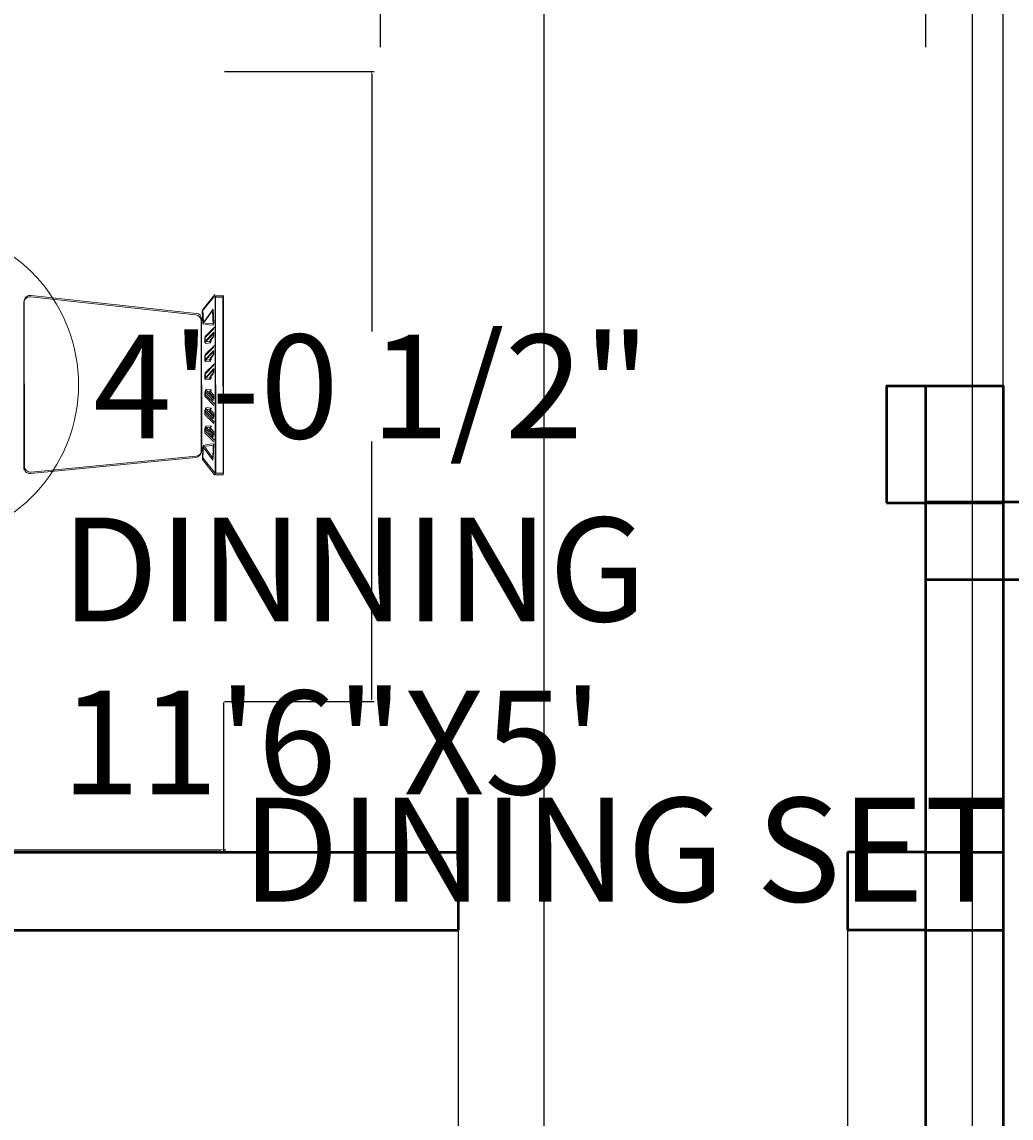
# Model space of a CAD drawing. Units: inches. Extents: x 1305 to 1889, y -508 to -5.
# Tile 5 of 8: x 1471 to 1548, y -305 to -220. Entities that reach past the tile are written whole.
import ezdxf

# ---------------------------------------------------------------- set-up
doc = ezdxf.new("R2010")
doc.units = ezdxf.units.IN
doc.header["$MEASUREMENT"] = 0
for name, color, linetype, lineweight in [('A-ANNO-DIMS', 2, 'Continuous', 18), ('A-AREA-IDEN', 7, 'Continuous', 25), ('A-COLS', 7, 'Continuous', 50), ('A-DOOR', 3, 'Continuous', 25), ('A-FURN', 8, 'Continuous', 18), ('A-WALL', 7, 'Continuous', 50)]:
    doc.layers.add(name, color=color, linetype=linetype, lineweight=lineweight)
doc.styles.get("Standard").update_dxf_attribs({"font": 'arial.ttf', "height": 8})
doc.dimstyles.get("Standard").update_dxf_attribs({"dimtxt": 0.18, "dimasz": 0.18, "dimexe": 0.18, "dimexo": 0.0625, "dimgap": 0.09, "dimtad": 0, "dimtih": 1, "dimtoh": 1, "dimzin": 0, "dimdsep": 46, "dimlunit": 4, "dimtxsty": 'Standard', "dimcen": 0.09, "dimadec": 0, "dimazin": 0, "dimtfac": 1, "dimtofl": 0, "dimtmove": 0, "dimatfit": 3, "dimfxl": 1, "dimtolj": 1, "dimtzin": 0, "dimarcsym": 0})

# ---------------------------------------------------------------- blocks, each defined once
blk = doc.blocks.new('A$C610239F1')
for p, q in [((2.0876, 1.0675, -0.0908), (2.5216, 1.0203, -0.0908)), ((2.5694, 1.0658, -0.0908), (2.5375, 1.0258, -0.0908)), ((2.5709, 1.0699, -0.0908), (2.539, 1.03, -0.0908)), ((2.5932, 1.0667, -0.0908), (2.5725, 1.0667, -0.0908)), ((2.5725, 1.0667, -0.0908), (2.5729, 0.6005, -0.0908)), ((2.5936, 0.6006, -0.0908), (2.5932, 1.0667, -0.0908)), ((2.0687, 0.6151, -0.0908), (2.0683, 1.0475, -0.0908)), ((2.0702, 0.6193, -0.0908), (2.0699, 1.0517, -0.0908)), ((2.086, 1.0634, -0.0908), (2.5201, 1.0162, -0.0908)), ((2.5917, 1.0626, -0.0908), (2.571, 1.0626, -0.0908)), ((2.571, 1.0626, -0.0908), (2.5714, 0.5964, -0.0908)), ((2.5921, 0.5964, -0.0908), (2.5917, 1.0626, -0.0908)), ((2.5375, 1.0258, -0.0908), (2.5391, 0.9923, -0.0908)), ((2.539, 1.03, -0.0908), (2.5406, 0.9964, -0.0908)), ((2.5391, 0.9923, -0.0908), (2.5646, 1.0275, -0.0908)), ((2.5406, 0.9964, -0.0908), (2.5661, 1.0316, -0.0908)), ((2.5646, 1.0275, -0.0908), (2.5663, 0.9892, -0.0908)), ((2.5661, 1.0316, -0.0908), (2.5678, 0.9933, -0.0908)), ((2.5343, 1.0004, -0.0908), (2.5346, 0.6572, -0.0908)), ((2.5358, 1.0045, -0.0908), (2.5361, 0.6613, -0.0908)), ((2.5663, 0.9892, -0.0908), (2.5439, 0.9907, -0.0908)), ((2.5679, 0.9796, -0.0908), (2.5439, 0.9556, -0.0908)), ((2.5678, 0.9933, -0.0908), (2.5454, 0.9948, -0.0908)), ((2.5694, 0.9837, -0.0908), (2.5455, 0.9597, -0.0908)), ((2.5439, 0.9556, -0.0908), (2.544, 0.9428, -0.0908)), ((2.544, 0.9428, -0.0908), (2.5663, 0.9668, -0.0908)), ((2.5455, 0.947, -0.0908), (2.5678, 0.9709, -0.0908)), ((2.5455, 0.9597, -0.0908), (2.5455, 0.947, -0.0908)), ((2.5663, 0.9572, -0.0908), (2.5567, 0.946, -0.0908)), ((2.5678, 0.9613, -0.0908), (2.5582, 0.9502, -0.0908)), ((2.5663, 0.9668, -0.0908), (2.5663, 0.9572, -0.0908)), ((2.5678, 0.9709, -0.0908), (2.5678, 0.9613, -0.0908)), ((2.5679, 0.9317, -0.0908), (2.544, 0.9077, -0.0908)), ((2.5694, 0.9358, -0.0908), (2.5455, 0.9118, -0.0908)), ((2.5455, 0.8991, -0.0908), (2.5678, 0.923, -0.0908)), ((2.5599, 0.9428, -0.0908), (2.5456, 0.9412, -0.0908)), ((2.5614, 0.947, -0.0908), (2.5471, 0.9454, -0.0908)), ((2.5567, 0.946, -0.0908), (2.5599, 0.9428, -0.0908)), ((2.5582, 0.9502, -0.0908), (2.5614, 0.947, -0.0908)), ((2.5678, 0.923, -0.0908), (2.5678, 0.9134, -0.0908)), ((2.544, 0.8949, -0.0908), (2.5663, 0.9189, -0.0908)), ((2.544, 0.9077, -0.0908), (2.544, 0.8949, -0.0908)), ((2.5455, 0.9118, -0.0908), (2.5455, 0.8991, -0.0908)), ((2.56, 0.895, -0.0908), (2.5456, 0.8933, -0.0908)), ((2.5615, 0.8991, -0.0908), (2.5471, 0.8975, -0.0908)), ((2.5663, 0.9093, -0.0908), (2.5568, 0.8981, -0.0908)), ((2.5568, 0.8981, -0.0908), (2.56, 0.895, -0.0908)), ((2.5678, 0.9134, -0.0908), (2.5583, 0.9023, -0.0908)), ((2.5583, 0.9023, -0.0908), (2.5615, 0.8991, -0.0908)), ((2.5663, 0.9189, -0.0908), (2.5663, 0.9093, -0.0908)), ((2.5679, 0.8838, -0.0908), (2.544, 0.8598, -0.0908)), ((2.544, 0.847, -0.0908), (2.5664, 0.871, -0.0908)), ((2.5695, 0.8879, -0.0908), (2.5455, 0.8639, -0.0908)), ((2.5456, 0.8512, -0.0908), (2.5679, 0.8751, -0.0908)), ((2.5679, 0.8656, -0.0908), (2.5583, 0.8544, -0.0908)), ((2.5664, 0.871, -0.0908), (2.5664, 0.8614, -0.0908)), ((2.5679, 0.8751, -0.0908), (2.5679, 0.8656, -0.0908)), ((2.544, 0.8598, -0.0908), (2.544, 0.847, -0.0908)), ((2.5455, 0.8639, -0.0908), (2.5456, 0.8512, -0.0908)), ((2.56, 0.8471, -0.0908), (2.5456, 0.8454, -0.0908)), ((2.5615, 0.8512, -0.0908), (2.5472, 0.8496, -0.0908)), ((2.5664, 0.8614, -0.0908), (2.5568, 0.8502, -0.0908)), ((2.5568, 0.8502, -0.0908), (2.56, 0.8471, -0.0908)), ((2.5583, 0.8544, -0.0908), (2.5615, 0.8512, -0.0908)), ((2.5441, 0.8023, -0.0908), (2.5441, 0.8151, -0.0908)), ((2.5441, 0.8151, -0.0908), (2.5664, 0.7912, -0.0908)), ((2.5456, 0.8065, -0.0908), (2.5456, 0.8192, -0.0908)), ((2.5456, 0.8192, -0.0908), (2.5679, 0.7953, -0.0908)), ((2.5695, 0.7825, -0.0908), (2.5456, 0.8065, -0.0908)), ((2.56, 0.8151, -0.0908), (2.5457, 0.8167, -0.0908)), ((2.5615, 0.8192, -0.0908), (2.5472, 0.8208, -0.0908)), ((2.5568, 0.8119, -0.0908), (2.56, 0.8151, -0.0908)), ((2.5664, 0.8008, -0.0908), (2.5568, 0.8119, -0.0908)), ((2.5583, 0.8161, -0.0908), (2.5615, 0.8192, -0.0908)), ((2.5679, 0.8049, -0.0908), (2.5583, 0.8161, -0.0908)), ((2.568, 0.7784, -0.0908), (2.5441, 0.8023, -0.0908)), ((2.5664, 0.7912, -0.0908), (2.5664, 0.8008, -0.0908)), ((2.5679, 0.7953, -0.0908), (2.5679, 0.8049, -0.0908)), ((2.5441, 0.7544, -0.0908), (2.5441, 0.7672, -0.0908)), ((2.5441, 0.7672, -0.0908), (2.5665, 0.7433, -0.0908)), ((2.5681, 0.7305, -0.0908), (2.5441, 0.7544, -0.0908)), ((2.5456, 0.7586, -0.0908), (2.5456, 0.7713, -0.0908)), ((2.5456, 0.7713, -0.0908), (2.568, 0.7474, -0.0908)), ((2.5696, 0.7346, -0.0908), (2.5456, 0.7586, -0.0908)), ((2.5601, 0.7672, -0.0908), (2.5457, 0.7688, -0.0908)), ((2.5616, 0.7714, -0.0908), (2.5472, 0.7729, -0.0908)), ((2.5569, 0.764, -0.0908), (2.5601, 0.7672, -0.0908)), ((2.5665, 0.7529, -0.0908), (2.5569, 0.764, -0.0908)), ((2.5584, 0.7682, -0.0908), (2.5616, 0.7714, -0.0908)), ((2.568, 0.757, -0.0908), (2.5584, 0.7682, -0.0908)), ((2.5665, 0.7433, -0.0908), (2.5665, 0.7529, -0.0908)), ((2.568, 0.7474, -0.0908), (2.568, 0.757, -0.0908)), ((2.5457, 0.7107, -0.0908), (2.5457, 0.7234, -0.0908)), ((2.5457, 0.7234, -0.0908), (2.568, 0.6995, -0.0908)), ((2.5601, 0.7193, -0.0908), (2.5457, 0.7209, -0.0908)), ((2.5616, 0.7235, -0.0908), (2.5473, 0.725, -0.0908)), ((2.5584, 0.7203, -0.0908), (2.5616, 0.7235, -0.0908)), ((2.568, 0.7091, -0.0908), (2.5584, 0.7203, -0.0908)), ((2.5442, 0.7066, -0.0908), (2.5442, 0.7193, -0.0908)), ((2.5442, 0.7193, -0.0908), (2.5665, 0.6954, -0.0908)), ((2.5681, 0.6826, -0.0908), (2.5442, 0.7066, -0.0908)), ((2.5696, 0.6867, -0.0908), (2.5457, 0.7107, -0.0908)), ((2.5569, 0.7161, -0.0908), (2.5601, 0.7193, -0.0908)), ((2.5665, 0.705, -0.0908), (2.5569, 0.7161, -0.0908)), ((2.5665, 0.6954, -0.0908), (2.5665, 0.705, -0.0908)), ((2.568, 0.6995, -0.0908), (2.568, 0.7091, -0.0908)), ((2.5378, 0.6363, -0.0908), (2.5394, 0.6698, -0.0908)), ((2.5394, 0.6404, -0.0908), (2.5409, 0.6739, -0.0908)), ((2.5394, 0.6698, -0.0908), (2.565, 0.6347, -0.0908)), ((2.5409, 0.6739, -0.0908), (2.5665, 0.6388, -0.0908)), ((2.5665, 0.673, -0.0908), (2.5442, 0.6714, -0.0908)), ((2.568, 0.6772, -0.0908), (2.5457, 0.6755, -0.0908)), ((2.565, 0.6347, -0.0908), (2.5665, 0.673, -0.0908)), ((2.5665, 0.6388, -0.0908), (2.568, 0.6772, -0.0908)), ((2.5202, 0.6413, -0.0908), (2.0862, 0.5993, -0.0908)), ((2.5217, 0.6454, -0.0908), (2.0877, 0.6034, -0.0908)), ((2.5698, 0.5964, -0.0908), (2.5378, 0.6363, -0.0908)), ((2.5713, 0.6005, -0.0908), (2.5394, 0.6404, -0.0908)), ((2.5714, 0.5964, -0.0908), (2.5921, 0.5964, -0.0908)), ((2.5729, 0.6005, -0.0908), (2.5936, 0.6006, -0.0908))]:
    blk.add_line(p, q)
for centre, radius, start, end in [((1.7963, 0.8331), 0.416, 279.1321, 80.8679), ((2.0858, 1.0517, -0.0908), 0.016, 83.7931, 180.0502), ((2.0843, 1.0475, -0.0908), 0.016, 83.7931, 180.0502), ((2.5184, 1.0003, -0.0908), 0.016, 0.0502, 83.7931), ((2.5199, 1.0045, -0.0908), 0.016, 0.0502, 83.7931), ((2.5187, 0.6572, -0.0908), 0.016, 275.5303, 0.0502), ((2.5202, 0.6613, -0.0908), 0.016, 275.5303, 0.0502), ((2.0847, 0.6152, -0.0908), 0.016, 180.0502, 275.5303), ((2.0862, 0.6193, -0.0908), 0.016, 180.0502, 275.5303)]:
    blk.add_arc(centre, radius, start, end)
blk = doc.blocks.new('*U14')
for p, q in [((-750, 0), (-750, -100)), ((0, 0), (0, -100))]:
    blk.add_line(p, q)
blk.add_lwpolyline([(0, 0), (0, 750), (-43.75, 750), (-43.75, 0)], close=True)
blk.add_arc((0, 0), 750, 90, 180)
blk = doc.blocks.new('COL-9X9')
blk.add_lwpolyline([(0, 0), (9, 0), (9, 9), (0, 9)], close=True)
blk = doc.blocks.new('*D40')
at = {"layer": 'A-ANNO-DIMS', "color": 0, "lineweight": -2, "transparency": 16777216}
for p, q in [((1410.934, -272.704), (1410.934, -284.232)), ((1487, -272.704), (1487, -284.232)), ((1411.114, -284.052), (1486.82, -284.052)), ((1487, -284.052), (1487.18, -284.052))]:
    blk.add_line(p, q, dxfattribs=at)
at = {"layer": 'A-ANNO-DIMS', "color": 0, "transparency": 16777216}
for points in [[(1411.114, -284.022), (1411.114, -284.082), (1410.934, -284.052)], [(1486.82, -284.022), (1486.82, -284.082), (1487, -284.052)]]:
    blk.add_solid(points, dxfattribs=at)
at = {"layer": 'Defpoints', "color": 0, "transparency": 16777216}
for p in [(1410.934, -272.642), (1487, -272.642), (1487, -284.052)]:
    blk.add_point(p, dxfattribs=at)
at = {"layer": 'A-ANNO-DIMS', "color": 0, "transparency": 16777216, "insert": (1531.234, -284.052), "char_height": 8, "attachment_point": 5}
blk.add_mtext('\\A1;DINING SET 6\'-4"', dxfattribs=at)
blk = doc.blocks.new('*D41')
at = {"layer": 'A-ANNO-DIMS', "color": 0, "lineweight": -2, "transparency": 16777216}
for p, q in [((1487.062, -224.071), (1498.589, -224.071)), ((1498.409, -224.251), (1498.409, -244.13)), ((1498.409, -272.462), (1498.409, -252.583)), ((1487.062, -272.642), (1498.589, -272.642))]:
    blk.add_line(p, q, dxfattribs=at)
at = {"layer": 'A-ANNO-DIMS', "color": 0, "transparency": 16777216}
for points in [[(1498.379, -224.251), (1498.439, -224.251), (1498.409, -224.071)], [(1498.379, -272.462), (1498.439, -272.462), (1498.409, -272.642)]]:
    blk.add_solid(points, dxfattribs=at)
at = {"layer": 'Defpoints', "color": 0, "transparency": 16777216}
for p in [(1487, -224.071), (1498.409, -224.071), (1487, -272.642)]:
    blk.add_point(p, dxfattribs=at)
at = {"layer": 'A-ANNO-DIMS', "color": 0, "transparency": 16777216, "insert": (1498.409, -248.357), "char_height": 8, "attachment_point": 5}
blk.add_mtext('\\A1;4\'-0 1/2"', dxfattribs=at)
blk = doc.blocks.new('*D55')
at = {"layer": 'A-ANNO-DIMS', "color": 0, "lineweight": -2, "transparency": 16777216}
for p, q in [((1511.679, -135.632), (1511.679, -493.256)), ((1544.679, -146.132), (1544.679, -493.256)), ((1511.859, -493.076), (1517.388, -493.076)), ((1544.499, -493.076), (1538.971, -493.076))]:
    blk.add_line(p, q, dxfattribs=at)
at = {"layer": 'A-ANNO-DIMS', "color": 0, "transparency": 16777216}
for points in [[(1511.859, -493.046), (1511.859, -493.106), (1511.679, -493.076)], [(1544.499, -493.046), (1544.499, -493.106), (1544.679, -493.076)]]:
    blk.add_solid(points, dxfattribs=at)
at = {"layer": 'Defpoints', "color": 0, "transparency": 16777216}
for p in [(1511.679, -135.569), (1544.679, -146.069), (1544.679, -493.076)]:
    blk.add_point(p, dxfattribs=at)
at = {"layer": 'A-ANNO-DIMS', "color": 0, "transparency": 16777216, "insert": (1528.179, -493.076), "char_height": 8, "attachment_point": 5}
blk.add_mtext('\\A1;2\'-9"', dxfattribs=at)
blk = doc.blocks.new('*D61')
at = {"layer": 'A-ANNO-DIMS', "color": 0, "lineweight": -2, "transparency": 16777216}
for p, q in [((1505.074, -290.301), (1505.074, -493.256)), ((1535.074, -290.301), (1535.074, -493.256)), ((1505.254, -493.076), (1509.283, -493.076)), ((1534.894, -493.076), (1530.866, -493.076))]:
    blk.add_line(p, q, dxfattribs=at)
at = {"layer": 'A-ANNO-DIMS', "color": 0, "transparency": 16777216}
for points in [[(1505.254, -493.046), (1505.254, -493.106), (1505.074, -493.076)], [(1534.894, -493.046), (1534.894, -493.106), (1535.074, -493.076)]]:
    blk.add_solid(points, dxfattribs=at)
at = {"layer": 'Defpoints', "color": 0, "transparency": 16777216}
for p in [(1505.074, -290.239), (1535.074, -290.239), (1535.074, -493.076)]:
    blk.add_point(p, dxfattribs=at)
at = {"layer": 'A-ANNO-DIMS', "color": 0, "transparency": 16777216, "insert": (1520.074, -493.076), "char_height": 8, "attachment_point": 5}
blk.add_mtext('\\A1;2\'-6"', dxfattribs=at)
blk = doc.blocks.new('*D62')
at = {"layer": 'A-ANNO-DIMS', "color": 0, "lineweight": -2, "transparency": 16777216}
for p, q in [((1505.012, -284.239), (1329.13, -284.239)), ((1329.31, -284.419), (1329.31, -290.059)), ((1505.012, -290.239), (1329.13, -290.239)), ((1329.31, -290.419), (1329.13, -290.419)), ((1329.31, -290.239), (1329.31, -290.419))]:
    blk.add_line(p, q, dxfattribs=at)
at = {"layer": 'A-ANNO-DIMS', "color": 0, "transparency": 16777216}
for points in [[(1329.28, -284.419), (1329.34, -284.419), (1329.31, -284.239)], [(1329.28, -290.059), (1329.34, -290.059), (1329.31, -290.239)]]:
    blk.add_solid(points, dxfattribs=at)
at = {"layer": 'Defpoints', "color": 0, "transparency": 16777216}
for p in [(1505.074, -284.239), (1329.31, -290.239), (1505.074, -290.239)]:
    blk.add_point(p, dxfattribs=at)
at = {"layer": 'A-ANNO-DIMS', "color": 0, "transparency": 16777216, "insert": (1318.407, -290.419), "char_height": 8, "attachment_point": 5}
blk.add_mtext('\\A1;0\'-6"', dxfattribs=at)
blk = doc.blocks.new('*D69')
at = {"layer": 'A-ANNO-DIMS', "color": 0, "lineweight": -2, "transparency": 16777216}
for p, q in [((1547.074, -377.176), (1547.074, -85.834)), ((1547.254, -86.014), (1576.418, -86.014)), ((1576.598, -377.176), (1576.598, -85.834)), ((1576.598, -86.014), (1576.778, -86.014))]:
    blk.add_line(p, q, dxfattribs=at)
at = {"layer": 'A-ANNO-DIMS', "color": 0, "transparency": 16777216}
for points in [[(1547.254, -85.984), (1547.254, -86.044), (1547.074, -86.014)], [(1576.418, -85.984), (1576.418, -86.044), (1576.598, -86.014)]]:
    blk.add_solid(points, dxfattribs=at)
at = {"layer": 'Defpoints', "color": 0, "transparency": 16777216}
for p in [(1576.598, -86.014), (1547.074, -377.239), (1576.598, -377.239)]:
    blk.add_point(p, dxfattribs=at)
at = {"layer": 'A-ANNO-DIMS', "color": 0, "transparency": 16777216, "insert": (1596.889, -86.014), "char_height": 8, "attachment_point": 5}
blk.add_mtext('\\A1;2\'-5 1/2"', dxfattribs=at)

msp = doc.modelspace()

# ---------------------------------------------------------------- linework, layer by layer
at = {"layer": 'A-WALL'}
for p, q in [((1541.074, -248.321), (1541.074, -389.239)), ((1547.074, -248.321), (1547.074, -389.239)), ((1541.074, -257.239), (1631.074, -257.239)), ((1541.074, -263.239), (1631.074, -263.239)), ((1394.074, -284.239), (1505.074, -284.239)), ((1505.074, -284.239), (1505.074, -290.239)), ((1541.074, -284.239), (1535.074, -284.239)), ((1535.074, -284.239), (1535.074, -290.239)), ((1541.074, -284.239), (1547.074, -284.239)), ((1394.074, -290.239), (1505.074, -290.239)), ((1541.074, -290.239), (1535.074, -290.239)), ((1541.074, -290.239), (1547.074, -290.239))]:
    msp.add_line(p, q, dxfattribs=at)

# ---------------------------------------------------------------- block references
at = {"layer": 'A-COLS'}
msp.add_blockref('COL-9X9', (1538.084, -257.32), dxfattribs=at)
at = {"layer": 'A-DOOR', "xscale": 0.056, "yscale": 0.056, "zscale": 0.056}
msp.add_blockref('*U14', (1541.074, -216.594), dxfattribs=at)
at = {"layer": 'A-FURN', "xscale": 29.3277177469152, "yscale": 29.3277177469152, "zscale": 29.3277177469152}
msp.add_blockref('A$C610239F1', (1410.934, -272.642, -0.999), dxfattribs=at)

# ---------------------------------------------------------------- texts
at = {"layer": 'A-AREA-IDEN', "insert": (1474.479, -258.456), "char_height": 8, "attachment_point": 1}
msp.add_mtext_dynamic_manual_height_columns('DINNING\\P11\'6"X5\'', width=69.27903, gutter_width=40, heights=[0], dxfattribs=at)

# ---------------------------------------------------------------- dimensions: what is measured, and where the dimension line sits
at = {"layer": 'A-ANNO-DIMS'}
for base, p1, p2, picture, middle in [((1576.598, -86.014), (1547.074, -377.239), (1576.598, -377.239), '*D69', (1596.889, -86.014)), ((1544.679, -493.076), (1511.679, -135.569), (1544.679, -146.069), '*D55', (1528.179, -493.076)), ((1535.074, -493.076), (1505.074, -290.239), (1535.074, -290.239), '*D61', (1520.074, -493.076))]:
    dim = msp.add_linear_dim(base=base, p1=p1, p2=p2, dimstyle='Standard', override={"dimdec": 1, "dimlfac": 1, "dimrnd": 0, "dimzin": 1, "dimdsep": 46, "dimlunit": 4, "dimfrac": 2}, dxfattribs=at)
    dim.commit()
    dim.dimension.update_dxf_attribs({"geometry": picture, "text_midpoint": middle})
for base, p1, p2, picture, middle in [((1498.409, -224.071), (1487, -272.642), (1487, -224.071), '*D41', (1498.409, -248.357)), ((1329.31, -290.239), (1505.074, -284.239), (1505.074, -290.239), '*D62', (1318.407, -290.419))]:
    dim = msp.add_linear_dim(base=base, p1=p1, p2=p2, angle=90, dimstyle='Standard', override={"dimdec": 1, "dimlfac": 1, "dimrnd": 0, "dimzin": 1, "dimdsep": 46, "dimlunit": 4, "dimfrac": 2}, dxfattribs=at)
    dim.commit()
    dim.dimension.update_dxf_attribs({"geometry": picture, "text_midpoint": middle})
dim = msp.add_linear_dim(base=(1487, -284.052), p1=(1410.934, -272.642), p2=(1487, -272.642), text='DINING SET <>', dimstyle='Standard', override={"dimdec": 1, "dimlfac": 1, "dimrnd": 0, "dimzin": 1, "dimdsep": 46, "dimlunit": 4, "dimfrac": 2}, dxfattribs=at)
dim.commit()
dim.dimension.update_dxf_attribs({"geometry": '*D40', "text_midpoint": (1531.234, -284.052)})

doc.saveas('drawing.dxf')
